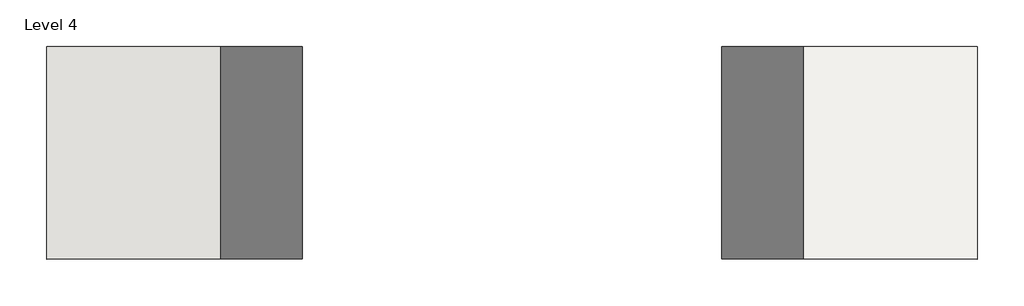
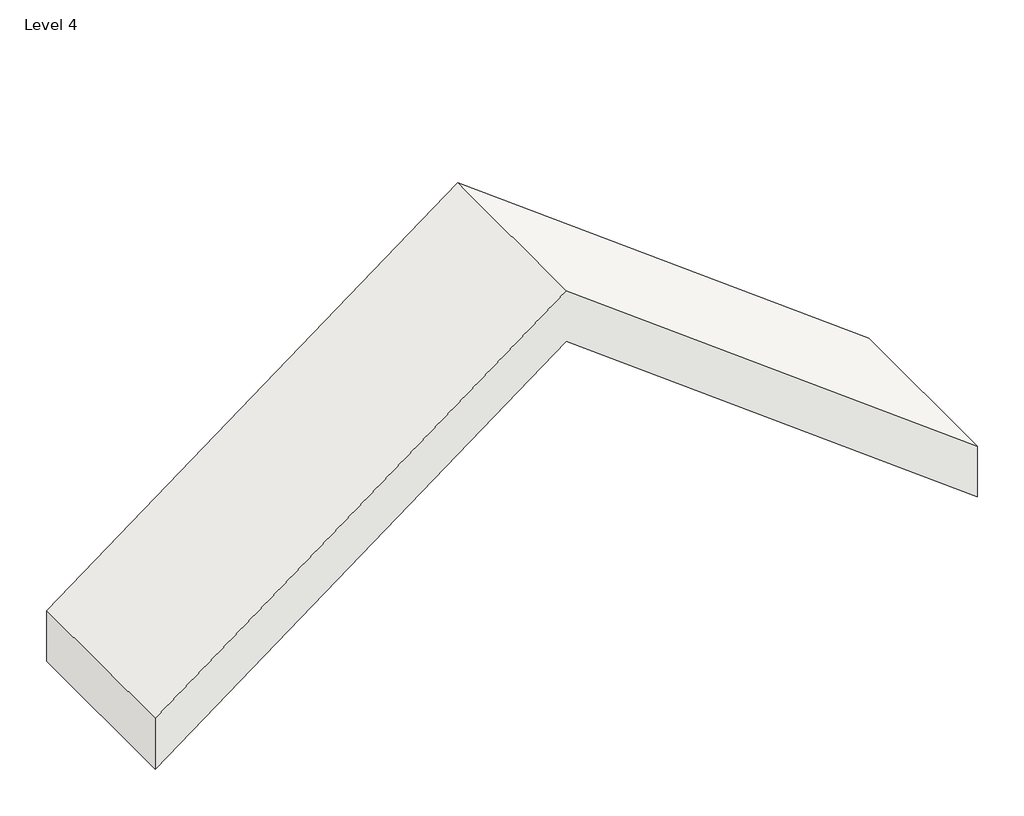
# One storey: 1 roof.
"""IFC4 building model written with IfcOpenShell, lengths in millimetres."""

from ifc_helpers import new_model, si_unit, frame, origin, place, context, project, spatial, polyline, outline, extrude, element, save

model = new_model("IFC4")

# Units and contexts
model_context = context("Model", 3, world=origin())
ifc_project = project(units=[si_unit("LENGTHUNIT", "METRE", prefix="MILLI")], contexts=[model_context])

# Site, building, storey
site = spatial("IfcSite", under=ifc_project)
building = spatial("IfcBuilding", under=site)
storey = spatial("IfcBuildingStorey", under=building, Name="Level 4", Elevation=9144.0)

# Roof
placement = place(None, origin())
element("IfcRoof", 1, ObjectType="Generic - 12\"", at=placement, inside=storey, context=model_context, shape_type="SweptSolid", body=[
    extrude(outline(polyline([(9525.0, -4635.4331929), (11710.9875, -7550.0831929), (9525.0, -10464.7331929), (9144.0, -10464.7331929), (11329.9875, -7550.0831929), (9144.0, -4635.4331929), (9525.0, -4635.4331929)])), frame((0.0, -10838.9092534, 0.0), z_axis=(0.0, 1.0, 0.0), x_axis=(0.0, 0.0, 1.0)), (0.0, 0.0, 1.0), 1333.5),
])

save(model, "model.ifc")

# Revit data of these elements
# Type "Generic - 12\""
#   Assembly Code = "B1020"
#   Layers, outside or top first: 1' - 0" no material (function 1)
# Element 1 (IfcRoof, "Generic - 12\"")
#   built-in parameter 1001705 = 38.4219 (stored number, unit not read)
#   built-in parameter 1001710 = 33615
#   Phase Created = New Construction
#   Materials on its faces: "Default Roof"
# Materials
#   "Default Roof": colour RGB 88 101 114, transparency 0, Cost = 0
